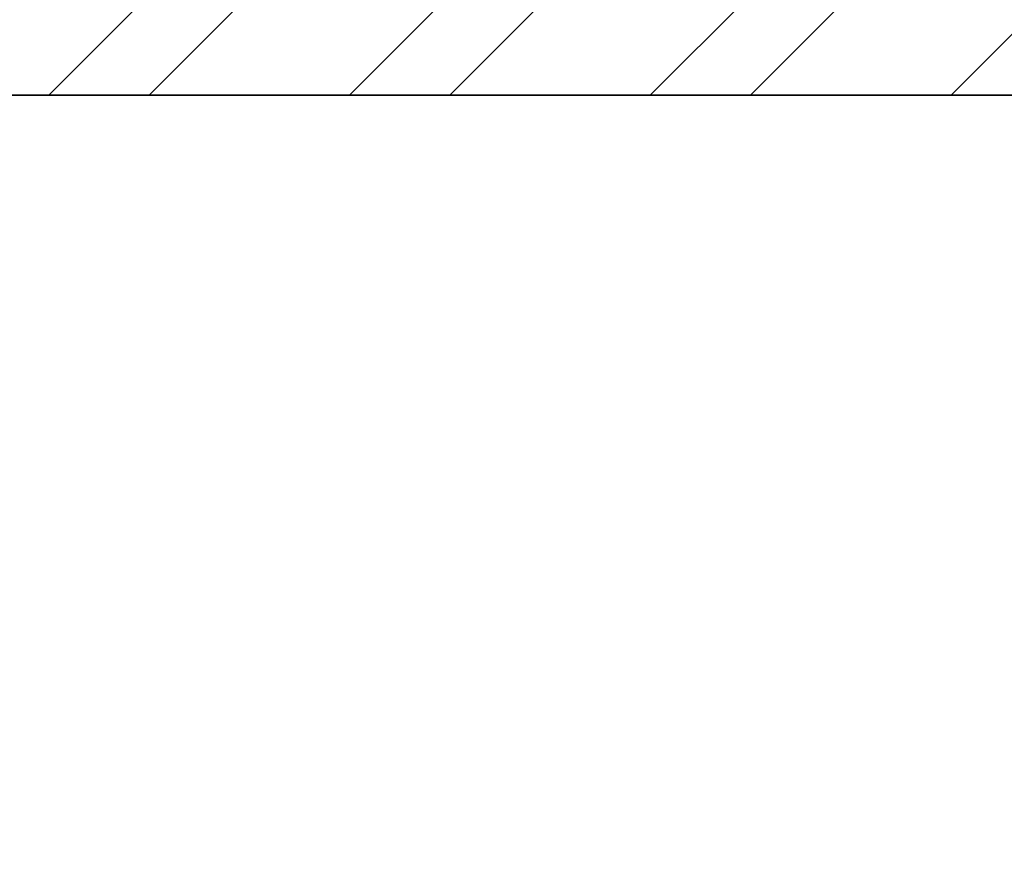
# Model space of a CAD drawing. Units: inches. Extents: x 1962 to 2771, y 1245 to 2660.
# Tile 30 of 114: x 2116 to 2160, y 1894 to 1932. Entities that reach past the tile are written whole.
import ezdxf

# ---------------------------------------------------------------- set-up
doc = ezdxf.new("R2010")
doc.units = ezdxf.units.IN
doc.layers.add('A-WALL', color=7, linetype='Continuous', lineweight=35)
doc.layers.add('A-WALL-PATT', color=252, linetype='Continuous', lineweight=13)

msp = doc.modelspace()

# ---------------------------------------------------------------- hatches: boundary and pattern name
at = {"layer": 'A-WALL-PATT'}
h = msp.add_hatch(dxfattribs=at)
h.set_pattern_fill('ANSI32', color=256)
h.paths.add_polyline_path([(2090.8074, 2467.3437), (2141.6481, 2467.3437), (2141.6481, 2469.5937), (2141.6481, 2471.8437), (2086.3074, 2471.8437), (2086.3074, 2422.5333), (2090.8074, 2422.5333)])
h.paths.add_polyline_path([(2282.7664, 2471.8437), (2204.8982, 2471.8437), (2204.8982, 2467.3437), (2234.8074, 2467.3437), (2234.8074, 2311.3437), (2228.7492, 2311.3437), (2228.7492, 2306.8437), (2234.8074, 2306.8437), (2331.9227, 2306.8437), (2331.9227, 2309.0937), (2331.9227, 2311.3437), (2239.3074, 2311.3437), (2239.3074, 2467.3437), (2282.7664, 2467.3437), (2282.7664, 2469.5937)])
h.paths.add_polyline_path([(2471.4531, 2519.8437), (2552.011, 2519.8437), (2564.3996, 2519.8437), (2564.3996, 2511.1389), (2568.8996, 2511.1389), (2568.8996, 2524.3437), (2466.9531, 2524.3437), (2466.9531, 2471.8437), (2450.0749, 2471.8437), (2446.4672, 2471.8437), (2446.4672, 2467.3437), (2450.0749, 2467.3437), (2475.9988, 2467.3437), (2475.9988, 2469.5937), (2475.9988, 2471.8437), (2471.4531, 2471.8437)])
h.paths.add_polyline_path([(2575.2231, 2469.5937), (2575.2231, 2471.8437), (2568.8996, 2471.8437), (2568.8996, 2487.1389), (2564.3996, 2487.1389), (2564.3996, 2471.8437), (2556.511, 2471.8437), (2499.2904, 2471.8437), (2499.2904, 2467.3437), (2507.8074, 2467.3437), (2507.8074, 2311.3437), (2414.863, 2311.3437), (2414.863, 2306.8437), (2512.3074, 2306.8437), (2517.0114, 2306.8437), (2517.0114, 2309.0937), (2517.0114, 2311.3437), (2512.3074, 2311.3437), (2512.3074, 2467.3437), (2575.2231, 2467.3437)])
h.paths.add_polyline_path([(2660.8074, 2471.8437), (2600.9602, 2471.8437), (2600.9602, 2467.3437), (2656.3074, 2467.3437), (2656.3074, 2432.5704), (2660.8074, 2432.5704)])
h.paths.add_polyline_path([(2660.8074, 2372.5704), (2656.3074, 2372.5704), (2656.3074, 2311.3437), (2600.276, 2311.3437), (2600.276, 2309.0937), (2600.276, 2306.8437), (2656.3074, 2306.8437), (2656.3074, 2296.2593), (2660.8074, 2296.2593)])
h.paths.add_polyline_path([(2572.3074, 2306.8437), (2577.1385, 2306.8437), (2577.1385, 2311.3437), (2551.082, 2311.3437), (2551.082, 2306.8437), (2567.8074, 2306.8437), (2567.8074, 2258.8437), (2540.0574, 2258.8437), (2540.0574, 2256.5937), (2540.0574, 2254.3437), (2567.8074, 2254.3437), (2656.3074, 2254.3437), (2656.3074, 2236.9085), (2660.8074, 2236.9085), (2660.8074, 2272.2593), (2656.3074, 2272.2593), (2656.3074, 2258.8437), (2572.3074, 2258.8437)])
h.paths.add_polyline_path([(2512.3074, 2254.3437), (2518.8716, 2254.3437), (2518.8716, 2256.5937), (2518.8716, 2258.8437), (2507.8074, 2258.8437), (2507.8074, 2177.8437), (2567.8074, 2177.8437), (2567.8074, 2172.9628), (2572.3074, 2172.9628), (2572.3074, 2177.8437), (2656.3074, 2177.8437), (2656.3074, 2166.4846), (2660.8074, 2166.4846), (2660.8074, 2200.9085), (2656.3074, 2200.9085), (2656.3074, 2182.3437), (2512.3074, 2182.3437)])
h.paths.add_polyline_path([(2656.3074, 2129.8437), (2572.3074, 2129.8437), (2572.3074, 2150.3044), (2570.0574, 2150.3044), (2567.8074, 2150.3044), (2567.8074, 2129.8437), (2507.8074, 2129.8437), (2507.8074, 2116.3027), (2510.0574, 2116.3027), (2512.3074, 2116.3027), (2512.3074, 2125.3437), (2567.8074, 2125.3437), (2572.3074, 2125.3437), (2656.3074, 2125.3437)])
h.paths.add_polyline_path([(2090.8074, 2362.5333), (2086.3074, 2362.5333), (2086.3074, 2298.6242), (2090.8074, 2298.6242), (2090.8074, 2306.8437), (2174.8074, 2306.8437), (2174.8074, 2286.4178), (2179.3074, 2286.4178), (2179.3074, 2306.8437), (2192.8641, 2306.8437), (2192.8641, 2309.0937), (2192.8641, 2311.3437), (2090.8074, 2311.3437)])
h.paths.add_polyline_path([(2209.156, 2258.8437), (2179.3074, 2258.8437), (2179.3074, 2263.2236), (2177.0574, 2263.2236), (2174.8074, 2263.2236), (2174.8074, 2258.8437), (2090.8074, 2258.8437), (2090.8074, 2274.6242), (2086.3074, 2274.6242), (2086.3074, 2238.2967), (2088.5574, 2238.2967), (2090.8074, 2238.2967), (2090.8074, 2254.3437), (2209.156, 2254.3437)])
h.paths.add_polyline_path([(2090.8074, 2177.8437), (2234.8074, 2177.8437), (2234.8074, 2173.1428), (2239.3074, 2173.1428), (2239.3074, 2258.8437), (2230.8442, 2258.8437), (2230.8442, 2256.5937), (2230.8442, 2254.3437), (2234.8074, 2254.3437), (2234.8074, 2182.3437), (2090.8074, 2182.3437), (2090.8074, 2202.2967), (2086.3074, 2202.2967), (2086.3074, 2140.0389), (2090.8074, 2140.0389)])
h.paths.add_polyline_path([(2090.8074, 2080.0389), (2086.3074, 2080.0389), (2086.3074, 2033.8437), (2090.8074, 2033.8437)], flags=17)
h.paths.add_polyline_path([(2244.9405, 2033.8437), (2239.3074, 2033.8437), (2239.3074, 2142.0665), (2237.2592, 2142.0665), (2234.8074, 2142.0665), (2234.8074, 2033.8437), (2090.8074, 2033.8437), (2076.5204, 2033.8437), (2072.0204, 2033.8437), (2072.0204, 2000.4493), (2076.5204, 2000.4493), (2076.5204, 2029.3437), (2090.8074, 2029.3437), (2244.9405, 2029.3437), (2244.9405, 2031.5937)])
h.paths.add_polyline_path([(2234.8074, 1933.3437), (2076.5204, 1933.3437), (2076.5204, 1952.4493), (2074.2704, 1952.4493), (2072.0204, 1952.4493), (2072.0204, 1933.3437), (2072.0204, 1928.8437), (2234.8074, 1928.8437)])
h.paths.add_polyline_path([(2090.8074, 1928.8437), (2086.3074, 1928.8437), (2086.3074, 1906.5013), (2090.8074, 1906.5013)])
h.paths.add_polyline_path([(2090.8074, 1846.5013), (2086.3074, 1846.5013), (2086.3074, 1769.9917), (2088.5574, 1769.9917), (2090.8074, 1769.9917), (2090.8074, 1780.3437), (2234.8074, 1780.3437), (2234.8074, 1708.3437), (2230.3764, 1708.3437), (2230.3764, 1703.8437), (2239.3074, 1703.8437), (2239.3074, 1792.6669), (2237.0574, 1792.6669), (2234.8074, 1792.6669), (2234.8074, 1784.8437), (2090.8074, 1784.8437)])
h.paths.add_polyline_path([(2239.3074, 1928.8437), (2244.9405, 1928.8437), (2244.9405, 1931.0937), (2244.9405, 1933.3437), (2234.8074, 1933.3437), (2234.8074, 1928.8437), (2234.8074, 1825.5949), (2239.3074, 1825.5949)])
h.paths.add_polyline_path([(2148.0425, 1649.0937), (2148.0425, 1651.3437), (2090.8074, 1651.3437), (2090.8074, 1646.8437), (2148.0425, 1646.8437)], flags=0)
h.paths.add_polyline_path([(2207.5601, 1708.3437), (2090.8074, 1708.3437), (2090.8074, 1703.8437), (2174.8074, 1703.8437), (2174.8074, 1651.3437), (2170.4457, 1651.3437), (2170.4457, 1646.8437), (2195.9924, 1646.8437), (2195.9924, 1649.0937), (2195.9924, 1651.3437), (2179.3074, 1651.3437), (2179.3074, 1703.8437), (2207.5601, 1703.8437), (2207.5601, 1706.0937)])
h.paths.add_polyline_path([(2090.8074, 1733.9917), (2086.3074, 1733.9917), (2086.3074, 1696.1032), (2088.5574, 1696.1032), (2090.8074, 1696.1032)])
h.paths.add_polyline_path([(2090.8074, 1672.1032), (2086.3074, 1672.1032), (2086.3074, 1600.3335), (2090.8074, 1600.3335)])
h.paths.add_polyline_path([(2090.8074, 1540.3335), (2086.3074, 1540.3335), (2086.3074, 1486.3437), (2139.6766, 1486.3437), (2139.6766, 1490.8437), (2090.8074, 1490.8437)])
h.paths.add_polyline_path([(2302.3876, 1490.8437), (2239.3074, 1490.8437), (2239.3074, 1646.8437), (2335.9994, 1646.8437), (2335.9994, 1651.3437), (2229.884, 1651.3437), (2229.884, 1646.8437), (2234.8074, 1646.8437), (2234.8074, 1490.8437), (2202.7103, 1490.8437), (2202.7103, 1488.5937), (2202.7103, 1486.3437), (2275.0699, 1486.3437), (2275.0699, 1475.772), (2279.5699, 1475.772), (2279.5699, 1486.3437), (2302.3876, 1486.3437)])
h.paths.add_polyline_path([(2279.5699, 1451.772), (2275.0699, 1451.772), (2275.0699, 1438.3437), (2174.8074, 1438.3437), (2174.8074, 1486.3437), (2179.7922, 1486.3437), (2179.7922, 1490.8437), (2163.3585, 1490.8437), (2163.3585, 1488.5937), (2163.3585, 1486.3437), (2170.3074, 1486.3437), (2170.3074, 1433.8437), (2279.5699, 1433.8437)])
h.paths.add_polyline_path([(2427.2363, 1490.8437), (2375.8074, 1490.8437), (2375.8074, 1646.8437), (2381.6401, 1646.8437), (2381.6401, 1651.3437), (2365.887, 1651.3437), (2365.887, 1649.0937), (2365.887, 1646.8437), (2371.3074, 1646.8437), (2371.3074, 1490.8437), (2327.5627, 1490.8437), (2327.5627, 1488.5937), (2327.5627, 1486.3437), (2371.3074, 1486.3437), (2371.3074, 1433.8437), (2375.8074, 1433.8437), (2375.8074, 1486.3437), (2427.2363, 1486.3437)])
h.paths.add_polyline_path([(2512.3074, 1646.8437), (2519.4351, 1646.8437), (2519.4351, 1649.0937), (2519.4351, 1651.3437), (2507.8074, 1651.3437), (2416.0063, 1651.3437), (2416.0063, 1649.0937), (2416.0063, 1646.8437), (2507.8074, 1646.8437), (2507.8074, 1490.8437), (2497.0532, 1490.8437), (2497.0532, 1488.5937), (2497.0532, 1486.3437), (2574.9344, 1486.3437), (2574.9344, 1476.0181), (2579.4344, 1476.0181), (2579.4344, 1486.3437), (2584.4872, 1486.3437), (2584.3074, 1490.8437), (2512.3074, 1490.8437)])
h.paths.add_polyline_path([(2470.5091, 1486.3437), (2473.9767, 1486.3437), (2473.9767, 1490.8437), (2449.6605, 1490.8437), (2449.6605, 1488.5937), (2449.6605, 1486.3437), (2466.0091, 1486.3437), (2466.0091, 1433.8437), (2470.5091, 1433.8437), (2579.4344, 1433.8437), (2579.4344, 1452.0181), (2574.9344, 1452.0181), (2574.9344, 1438.3437), (2554.5091, 1438.3437), (2470.5091, 1438.3437)])
h.paths.add_polyline_path([(2656.3074, 1490.8437), (2611.86, 1490.8437), (2611.86, 1486.3437), (2656.3074, 1486.3437)])
h.paths.add_polyline_path([(2660.8074, 1532.7007), (2658.5574, 1532.7007), (2656.3074, 1532.7007), (2656.3074, 1486.3437), (2660.8074, 1486.3437)])
h.paths.add_polyline_path([(2660.8074, 1664.9663), (2656.3074, 1664.9663), (2656.3074, 1651.3437), (2602.2313, 1651.3437), (2602.2313, 1646.8437), (2656.3074, 1646.8437), (2656.3074, 1592.7007), (2660.8074, 1592.7007)])
h.paths.add_polyline_path([(2660.8074, 1724.5221), (2656.3074, 1724.5221), (2656.3074, 1703.8437), (2542.4725, 1703.8437), (2542.4725, 1699.3437), (2567.8074, 1699.3437), (2567.8074, 1651.3437), (2552.7766, 1651.3437), (2552.7766, 1649.0937), (2552.7766, 1646.8437), (2577.2878, 1646.8437), (2577.2878, 1649.0937), (2577.2878, 1651.3437), (2572.3074, 1651.3437), (2572.3074, 1699.3437), (2656.3074, 1699.3437), (2656.3074, 1688.9663), (2660.8074, 1688.9663)])
h.paths.add_polyline_path([(2660.8074, 1880.6524), (2656.3074, 1880.6524), (2656.3074, 1832.8437), (2512.3074, 1832.8437), (2512.3074, 1837.8959), (2507.8074, 1837.8959), (2507.8074, 1828.3437), (2567.8074, 1828.3437), (2567.8074, 1804.3437), (2572.3074, 1804.3437), (2572.3074, 1828.3437), (2656.3074, 1828.3437), (2656.3074, 1818.6778), (2660.8074, 1818.6778)])
h.paths.add_polyline_path([(2660.8074, 1794.6778), (2656.3074, 1794.6778), (2656.3074, 1780.3437), (2572.3074, 1780.3437), (2572.3074, 1783.0303), (2570.0574, 1783.0303), (2567.8074, 1783.0303), (2567.8074, 1780.3437), (2507.8074, 1780.3437), (2507.8074, 1699.3437), (2517.8858, 1699.3437), (2517.8858, 1701.5937), (2517.8858, 1703.8437), (2512.3074, 1703.8437), (2512.3074, 1775.8437), (2656.3074, 1775.8437), (2656.3074, 1760.5221), (2660.8074, 1760.5221)])
h.paths.add_polyline_path([(2660.8074, 1981.3437), (2660.8074, 2020.2808), (2658.5574, 2020.2808), (2656.3074, 2020.2808), (2656.3074, 1981.3437), (2512.3074, 1981.3437), (2512.3074, 2086.6996), (2507.8074, 2086.6996), (2507.8074, 1981.3437), (2375.8074, 1981.3437), (2375.8074, 1986.8505), (2373.5574, 1986.8505), (2371.3074, 1986.8505), (2371.3074, 1973.2607), (2375.8074, 1973.2607), (2375.8074, 1976.8437), (2507.8074, 1976.8437), (2507.8074, 1865.4281), (2510.0574, 1865.4281), (2512.3074, 1865.4281), (2512.3074, 1976.8437), (2660.8074, 1976.8437)])
h.paths.add_polyline_path([(2375.8074, 1940.297), (2373.5574, 1940.297), (2371.3074, 1940.297), (2371.3074, 1933.3437), (2278.4434, 1933.3437), (2278.4434, 1928.8437), (2371.3074, 1928.8437), (2371.3074, 1651.3437), (2375.8074, 1651.3437)])
h.paths.add_polyline_path([(2660.8074, 1976.8437), (2656.3074, 1976.8437), (2656.3074, 1940.6524), (2660.8074, 1940.6524)], flags=17)
h.paths.add_polyline_path([(2660.8074, 2142.4846), (2656.3074, 2142.4846), (2656.3074, 2080.2808), (2660.8074, 2080.2808)])
h.paths.add_polyline_path([(2381.4189, 2311.3437), (2375.8074, 2311.3437), (2375.8074, 2467.3437), (2424.7242, 2467.3437), (2424.7242, 2469.5937), (2424.7242, 2471.8437), (2375.8074, 2471.8437), (2375.8074, 2524.3437), (2371.3074, 2524.3437), (2371.3074, 2471.8437), (2307.2097, 2471.8437), (2307.2097, 2467.3437), (2371.3074, 2467.3437), (2371.3074, 2311.3437), (2366.8901, 2311.3437), (2366.8901, 2306.8437), (2371.3074, 2306.8437), (2371.3074, 2033.8437), (2279.6589, 2033.8437), (2279.6589, 2029.3437), (2371.3074, 2029.3437), (2371.3074, 2014.2598), (2375.8074, 2014.2598), (2375.8074, 2306.8437), (2381.4189, 2306.8437)])
h.paths.add_polyline_path([(2263.3074, 2524.3437), (2170.3074, 2524.3437), (2170.3074, 2519.8437), (2170.3074, 2471.8437), (2165.0312, 2471.8437), (2165.0312, 2467.3437), (2179.6721, 2467.3437), (2179.6721, 2469.5161), (2179.6721, 2471.8437), (2174.8074, 2471.8437), (2174.8074, 2519.8437), (2258.8074, 2519.8437), (2258.8074, 2511.6436), (2263.3074, 2511.6436)])
h.paths.add_polyline_path([(2245.0232, 1361.4123), (2492.9468, 1361.4123), (2492.9468, 1398.505), (2245.0232, 1398.505)], flags=9)
h.paths.add_polyline_path([(2388.1434, 2086.6936), (2425.0704, 2086.6936), (2425.0704, 2105.3509), (2388.1434, 2105.3509)], flags=9)
h.paths.add_polyline_path([(2404.922, 2242.6744), (2445.7337, 2242.6744), (2445.7337, 2261.3318), (2404.922, 2261.3318)], flags=9)
h.paths.add_polyline_path([(2269.4107, 2156.7935), (2306.3378, 2156.7935), (2306.3378, 2175.4508), (2269.4107, 2175.4508)], flags=9)
h.paths.add_polyline_path([(2269.3277, 2233.4343), (2306.2547, 2233.4343), (2306.2547, 2252.0917), (2269.3277, 2252.0917)], flags=9)
h.paths.add_polyline_path([(2431.6052, 2320.6922), (2470.4456, 2320.6922), (2470.4456, 2339.3495), (2431.6052, 2339.3495)], flags=25)
h.paths.add_polyline_path([(2249.6902, 2315.7608), (2288.5306, 2315.7608), (2288.5306, 2334.4182), (2249.6902, 2334.4182)], flags=25)
h.paths.add_polyline_path([(2096.9301, 2314.3181), (2135.7704, 2314.3181), (2135.7704, 2332.9755), (2096.9301, 2332.9755)], flags=25)
h.paths.add_polyline_path([(2134.3475, 2285.7089), (2161.4655, 2285.7089), (2161.4655, 2304.3662), (2134.3475, 2304.3662)], flags=9)
h.paths.add_polyline_path([(2126.5155, 2209.4076), (2159.9227, 2209.4076), (2159.9227, 2228.065), (2126.5155, 2228.065)], flags=25)
h.paths.add_polyline_path([(2110.5753, 2141.5299), (2149.4157, 2141.5299), (2149.4157, 2160.1872), (2110.5753, 2160.1872)], flags=25)
h.paths.add_polyline_path([(2249.8618, 1968.3317), (2286.3966, 1968.3317), (2286.3966, 1986.989), (2249.8618, 1986.989)], flags=9)
h.paths.add_polyline_path([(2395.9507, 1777.0051), (2436.7624, 1777.0051), (2436.7624, 1795.6625), (2395.9507, 1795.6625)], flags=9)
h.paths.add_polyline_path([(2398.5259, 1888.5651), (2435.0062, 1888.5651), (2435.0062, 1907.2224), (2398.5259, 1907.2224)], flags=25)
h.paths.add_polyline_path([(2259.3506, 1728.3559), (2296.2776, 1728.3559), (2296.2776, 1747.0132), (2259.3506, 1747.0132)], flags=9)
h.paths.add_polyline_path([(2271.3698, 1845.268), (2308.2968, 1845.268), (2308.2968, 1863.9253), (2271.3698, 1863.9253)], flags=9)
h.paths.add_polyline_path([(2120.9355, 1786.3027), (2159.7759, 1786.3027), (2159.7759, 1804.9601), (2120.9355, 1804.9601)], flags=25)
h.paths.add_polyline_path([(2121.3164, 1732.1043), (2154.7236, 1732.1043), (2154.7236, 1750.7616), (2121.3164, 1750.7616)], flags=25)
h.paths.add_polyline_path([(2118.3706, 1678.8997), (2147.5282, 1678.8997), (2147.5282, 1697.557), (2118.3706, 1697.557)], flags=25)
h.paths.add_polyline_path([(2385.9227, 1493.557), (2424.763, 1493.557), (2424.763, 1512.2143), (2385.9227, 1512.2143)], flags=25)
h.paths.add_polyline_path([(2248.7058, 1500.0256), (2287.5462, 1500.0256), (2287.5462, 1518.6829), (2248.7058, 1518.6829)], flags=25)
h.paths.add_polyline_path([(2104.1669, 1617.3771), (2143.0073, 1617.3771), (2143.0073, 1636.0344), (2104.1669, 1636.0344)], flags=9)
h.paths.add_polyline_path([(2096.0714, 1447.8824), (2137.3845, 1447.8824), (2137.3845, 1458.1859), (2096.0714, 1458.1859)], flags=9)
h.paths.add_polyline_path([(2180.6114, 1440.325), (2209.7689, 1440.325), (2209.7689, 1458.9823), (2180.6114, 1458.9823)], flags=25)
h.paths.add_polyline_path([(2316.1698, 1447.9637), (2357.4829, 1447.9637), (2357.4829, 1458.2673), (2316.1698, 1458.2673)], flags=9)
h.paths.add_polyline_path([(2397.6187, 1447.9637), (2438.9318, 1447.9637), (2438.9318, 1458.2673), (2397.6187, 1458.2673)], flags=9)
h.paths.add_polyline_path([(2473.0778, 1439.5953), (2502.2354, 1439.5953), (2502.2354, 1458.2527), (2473.0778, 1458.2527)], flags=25)
h.paths.add_polyline_path([(2589.7027, 1447.8819), (2631.0158, 1447.8819), (2631.0158, 1458.1855), (2589.7027, 1458.1855)], flags=9)
h.paths.add_polyline_path([(2522.4009, 1497.5285), (2561.2413, 1497.5285), (2561.2413, 1516.1859), (2522.4009, 1516.1859)], flags=25)
h.paths.add_polyline_path([(2579.6565, 1671.3482), (2608.8141, 1671.3482), (2608.8141, 1690.0056), (2579.6565, 1690.0056)], flags=25)
h.paths.add_polyline_path([(2544.7038, 1725.5064), (2578.1111, 1725.5064), (2578.1111, 1744.1637), (2544.7038, 1744.1637)], flags=25)
h.paths.add_polyline_path([(2578.1191, 1807.472), (2607.2766, 1807.472), (2607.2766, 1826.1293), (2578.1191, 1826.1293)], flags=25)
h.paths.add_polyline_path([(2595.0614, 1835.1839), (2633.9018, 1835.1839), (2633.9018, 1853.8413), (2595.0614, 1853.8413)], flags=25)
h.paths.add_polyline_path([(2567.0097, 2097.7035), (2605.8501, 2097.7035), (2605.8501, 2116.3609), (2567.0097, 2116.3609)], flags=9)
h.paths.add_polyline_path([(2586.644, 2134.6454), (2615.8015, 2134.6454), (2615.8015, 2153.3027), (2586.644, 2153.3027)], flags=9)
h.paths.add_polyline_path([(2544.6185, 2212.6783), (2578.0258, 2212.6783), (2578.0258, 2231.3356), (2544.6185, 2231.3356)], flags=25)
h.paths.add_polyline_path([(2577.0273, 2256.9023), (2606.1849, 2256.9023), (2606.1849, 2275.5597), (2577.0273, 2275.5597)], flags=24)
h.paths.add_polyline_path([(2605.2683, 2315.2821), (2644.1087, 2315.2821), (2644.1087, 2333.9395), (2605.2683, 2333.9395)], flags=25)
h.paths.add_polyline_path([(2583.1244, 2496.1815), (2624.4375, 2496.1815), (2624.4375, 2506.4851), (2583.1244, 2506.4851)], flags=9)
h.paths.add_polyline_path([(2474.761, 2497.0823), (2503.9185, 2497.0823), (2503.9185, 2515.7397), (2474.761, 2515.7397)], flags=25)
h.paths.add_polyline_path([(2387.5787, 2494.2563), (2428.902, 2494.2563), (2428.902, 2504.5598), (2387.5787, 2504.5598)], flags=9)
h.paths.add_polyline_path([(2300.1657, 2500.1564), (2341.4788, 2500.1564), (2341.4788, 2510.46), (2300.1657, 2510.46)], flags=25)
h.paths.add_polyline_path([(2176.8589, 2497.5843), (2206.0165, 2497.5843), (2206.0165, 2516.2416), (2176.8589, 2516.2416)], flags=25)
h.paths.add_polyline_path([(2097.4668, 2494.9762), (2138.7799, 2494.9762), (2138.7799, 2505.2798), (2097.4668, 2505.2798)], flags=9)

# ---------------------------------------------------------------- linework, layer by layer
at = {"layer": 'A-WALL'}
msp.add_line((2072.0204, 1928.8437), (2234.8074, 1928.8437), dxfattribs=at)

doc.saveas('drawing.dxf')
